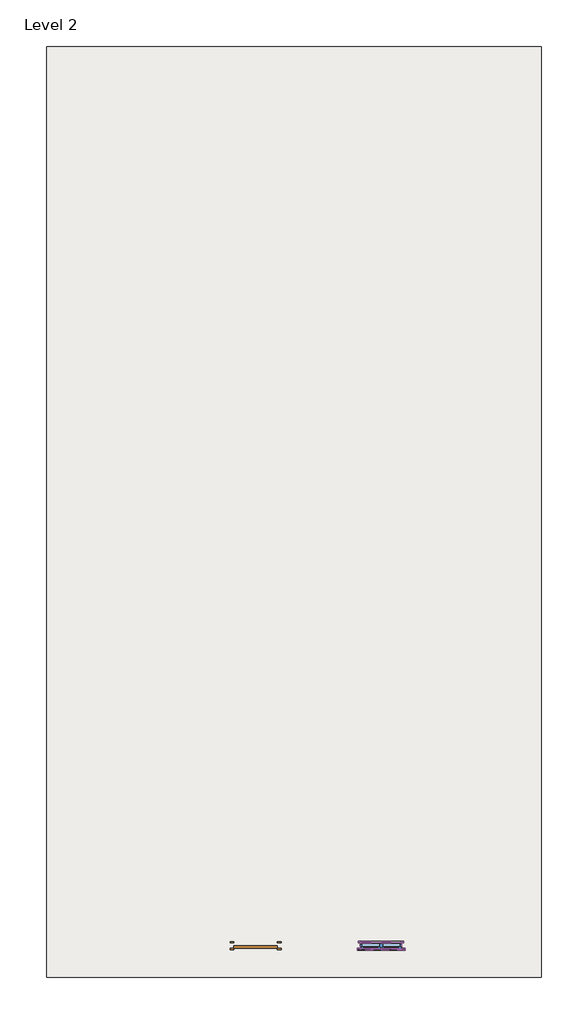
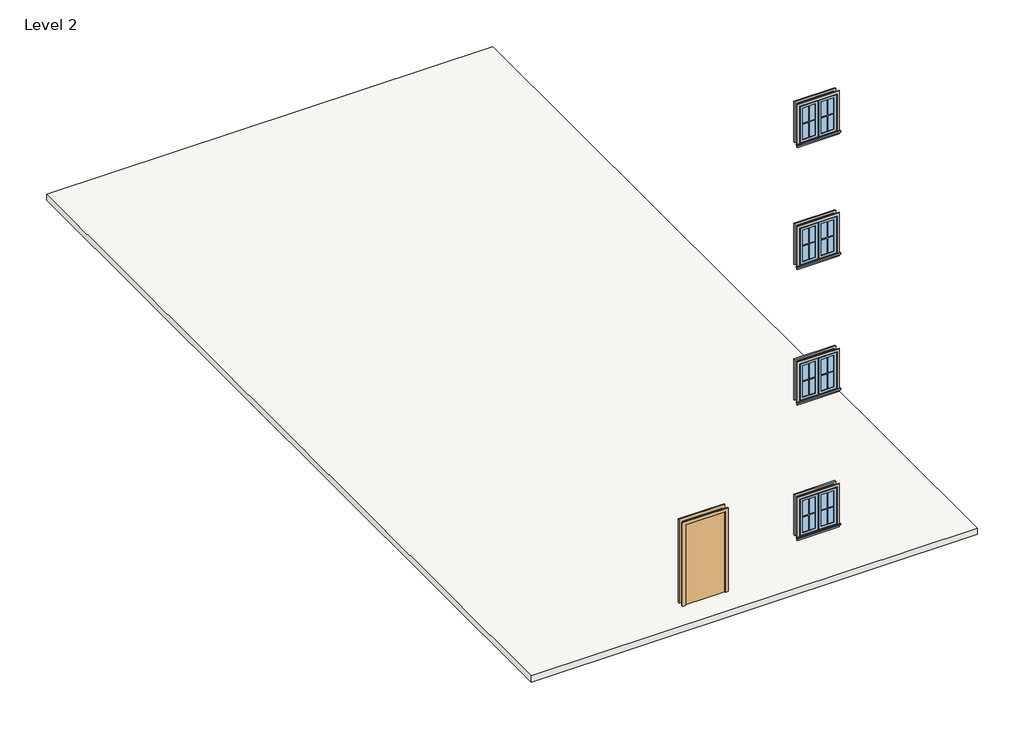
# One storey, incomplete: 16 proxies, 4 windows, 1 door, 1 roof.
"""IFC4 building model written with IfcOpenShell, lengths in millimetres."""

from ifc_helpers import new_model, si_unit, frame, origin, place, context, project, spatial, polyline, outline, extrude, transform, mapped, element, save
from components import muntin_pattern_2x2_muntin_pattern_2x2_b3fe6957, muntin_pattern_2x2_muntin_pattern_2x2_3e0ecaf2, trim_window_exterior_flat_with_sill_41619996, trim_window_interior_flat_picture_frame_51c85655, door_e5f9f3c4, window_a598f463

model = new_model("IFC4")

# Units and contexts
model_context = context("Model", 3, world=origin())
ifc_project = project(units=[si_unit("LENGTHUNIT", "METRE", prefix="MILLI")], contexts=[model_context])

# Site, building, storey
site = spatial("IfcSite", under=ifc_project)
building = spatial("IfcBuilding", under=site)
storey = spatial("IfcBuildingStorey", under=building, Name="Level 2", Elevation=3048.0)

# Proxies
placement = place(None, origin())
muntin_pattern_2x2_muntin_pattern_2x2_shape = muntin_pattern_2x2_muntin_pattern_2x2_b3fe6957(model_context)
element("IfcBuildingElementProxy", 1, Name="Muntin Pattern_2x2 : Muntin Pattern_2x2", ObjectType="Muntin Pattern_2x2 : Muntin Pattern_2x2", at=placement, inside=storey, context=model_context, shape_type="MappedRepresentation", body=[
    mapped(muntin_pattern_2x2_muntin_pattern_2x2_shape, transform((787.8709916, -7851.4177733, 4032.25), x_axis=(-1.0, 0.0, 0.0), y_axis=(0.0, -1.0, 0.0), z_axis=(0.0, 0.0, 1.0))),
])
element("IfcBuildingElementProxy", 2, Name="Muntin Pattern_2x2 : Muntin Pattern_2x2", ObjectType="Muntin Pattern_2x2 : Muntin Pattern_2x2", at=placement, inside=storey, context=model_context, shape_type="MappedRepresentation", body=[
    mapped(muntin_pattern_2x2_muntin_pattern_2x2_shape, transform((787.8709916, -7851.4177733, 7355.1690366), x_axis=(-1.0, 0.0, 0.0), y_axis=(0.0, -1.0, 0.0), z_axis=(0.0, 0.0, 1.0))),
])
element("IfcBuildingElementProxy", 3, Name="Muntin Pattern_2x2 : Muntin Pattern_2x2", ObjectType="Muntin Pattern_2x2 : Muntin Pattern_2x2", at=placement, inside=storey, context=model_context, shape_type="MappedRepresentation", body=[
    mapped(muntin_pattern_2x2_muntin_pattern_2x2_shape, transform((787.8709916, -7851.4177733, 10685.2522943), x_axis=(-1.0, 0.0, 0.0), y_axis=(0.0, -1.0, 0.0), z_axis=(0.0, 0.0, 1.0))),
])
element("IfcBuildingElementProxy", 4, Name="Muntin Pattern_2x2 : Muntin Pattern_2x2", ObjectType="Muntin Pattern_2x2 : Muntin Pattern_2x2", at=placement, inside=storey, context=model_context, shape_type="MappedRepresentation", body=[
    mapped(muntin_pattern_2x2_muntin_pattern_2x2_shape, transform((787.8709916, -7851.4177733, 13681.7979476), x_axis=(-1.0, 0.0, 0.0), y_axis=(0.0, -1.0, 0.0), z_axis=(0.0, 0.0, 1.0))),
])
muntin_pattern_2x2_muntin_pattern_2x2_2_shape = muntin_pattern_2x2_muntin_pattern_2x2_3e0ecaf2(model_context)
element("IfcBuildingElementProxy", 5, Name="Muntin Pattern_2x2 : Muntin Pattern_2x2", ObjectType="Muntin Pattern_2x2 : Muntin Pattern_2x2", at=placement, inside=storey, context=model_context, shape_type="MappedRepresentation", body=[
    mapped(muntin_pattern_2x2_muntin_pattern_2x2_2_shape, transform((359.2459916, -7851.4177733, 4032.25), x_axis=(1.0, 0.0, 0.0), y_axis=(0.0, 1.0, 0.0), z_axis=(0.0, 0.0, 1.0))),
])
element("IfcBuildingElementProxy", 6, Name="Muntin Pattern_2x2 : Muntin Pattern_2x2", ObjectType="Muntin Pattern_2x2 : Muntin Pattern_2x2", at=placement, inside=storey, context=model_context, shape_type="MappedRepresentation", body=[
    mapped(muntin_pattern_2x2_muntin_pattern_2x2_2_shape, transform((359.2459916, -7851.4177733, 7355.1690366), x_axis=(1.0, 0.0, 0.0), y_axis=(0.0, 1.0, 0.0), z_axis=(0.0, 0.0, 1.0))),
])
element("IfcBuildingElementProxy", 7, Name="Muntin Pattern_2x2 : Muntin Pattern_2x2", ObjectType="Muntin Pattern_2x2 : Muntin Pattern_2x2", at=placement, inside=storey, context=model_context, shape_type="MappedRepresentation", body=[
    mapped(muntin_pattern_2x2_muntin_pattern_2x2_2_shape, transform((359.2459916, -7851.4177733, 10685.2522943), x_axis=(1.0, 0.0, 0.0), y_axis=(0.0, 1.0, 0.0), z_axis=(0.0, 0.0, 1.0))),
])
element("IfcBuildingElementProxy", 8, Name="Muntin Pattern_2x2 : Muntin Pattern_2x2", ObjectType="Muntin Pattern_2x2 : Muntin Pattern_2x2", at=placement, inside=storey, context=model_context, shape_type="MappedRepresentation", body=[
    mapped(muntin_pattern_2x2_muntin_pattern_2x2_2_shape, transform((359.2459916, -7851.4177733, 13681.7979476), x_axis=(1.0, 0.0, 0.0), y_axis=(0.0, 1.0, 0.0), z_axis=(0.0, 0.0, 1.0))),
])
trim_window_exterior_flat_with_sill_shape = trim_window_exterior_flat_with_sill_41619996(model_context)
element("IfcBuildingElementProxy", 9, Name="Trim-Window-Exterior-Flat : with Sill", ObjectType="Trim-Window-Exterior-Flat : with Sill", at=placement, inside=storey, context=model_context, shape_type="MappedRepresentation", body=[
    mapped(trim_window_exterior_flat_with_sill_shape, transform((573.5584916, -7860.9427733, 4876.8), x_axis=(1.0, 0.0, 0.0), y_axis=(0.0, 0.0, 1.0), z_axis=(0.0, -1.0, 0.0))),
])
element("IfcBuildingElementProxy", 10, Name="Trim-Window-Exterior-Flat : with Sill", ObjectType="Trim-Window-Exterior-Flat : with Sill", at=placement, inside=storey, context=model_context, shape_type="MappedRepresentation", body=[
    mapped(trim_window_exterior_flat_with_sill_shape, transform((573.5584916, -7860.9427733, 8199.7190366), x_axis=(1.0, 0.0, 0.0), y_axis=(0.0, 0.0, 1.0), z_axis=(0.0, -1.0, 0.0))),
])
element("IfcBuildingElementProxy", 11, Name="Trim-Window-Exterior-Flat : with Sill", ObjectType="Trim-Window-Exterior-Flat : with Sill", at=placement, inside=storey, context=model_context, shape_type="MappedRepresentation", body=[
    mapped(trim_window_exterior_flat_with_sill_shape, transform((573.5584916, -7860.9427733, 11529.8022943), x_axis=(1.0, 0.0, 0.0), y_axis=(0.0, 0.0, 1.0), z_axis=(0.0, -1.0, 0.0))),
])
element("IfcBuildingElementProxy", 12, Name="Trim-Window-Exterior-Flat : with Sill", ObjectType="Trim-Window-Exterior-Flat : with Sill", at=placement, inside=storey, context=model_context, shape_type="MappedRepresentation", body=[
    mapped(trim_window_exterior_flat_with_sill_shape, transform((573.5584916, -7860.9427733, 14526.3479476), x_axis=(1.0, 0.0, 0.0), y_axis=(0.0, 0.0, 1.0), z_axis=(0.0, -1.0, 0.0))),
])
trim_window_interior_flat_picture_frame_shape = trim_window_interior_flat_picture_frame_51c85655(model_context)
element("IfcBuildingElementProxy", 13, Name="Trim-Window-Interior-Flat : Picture Frame", ObjectType="Trim-Window-Interior-Flat : Picture Frame", at=placement, inside=storey, context=model_context, shape_type="MappedRepresentation", body=[
    mapped(trim_window_interior_flat_picture_frame_shape, transform((573.5584916, -7746.6427733, 4876.8), x_axis=(-1.0, 0.0, 0.0), y_axis=(0.0, 0.0, 1.0), z_axis=(0.0, 1.0, 0.0))),
])
element("IfcBuildingElementProxy", 14, Name="Trim-Window-Interior-Flat : Picture Frame", ObjectType="Trim-Window-Interior-Flat : Picture Frame", at=placement, inside=storey, context=model_context, shape_type="MappedRepresentation", body=[
    mapped(trim_window_interior_flat_picture_frame_shape, transform((573.5584916, -7746.6427733, 8199.7190366), x_axis=(-1.0, 0.0, 0.0), y_axis=(0.0, 0.0, 1.0), z_axis=(0.0, 1.0, 0.0))),
])
element("IfcBuildingElementProxy", 15, Name="Trim-Window-Interior-Flat : Picture Frame", ObjectType="Trim-Window-Interior-Flat : Picture Frame", at=placement, inside=storey, context=model_context, shape_type="MappedRepresentation", body=[
    mapped(trim_window_interior_flat_picture_frame_shape, transform((573.5584916, -7746.6427733, 11529.8022943), x_axis=(-1.0, 0.0, 0.0), y_axis=(0.0, 0.0, 1.0), z_axis=(0.0, 1.0, 0.0))),
])
element("IfcBuildingElementProxy", 16, Name="Trim-Window-Interior-Flat : Picture Frame", ObjectType="Trim-Window-Interior-Flat : Picture Frame", at=placement, inside=storey, context=model_context, shape_type="MappedRepresentation", body=[
    mapped(trim_window_interior_flat_picture_frame_shape, transform((573.5584916, -7746.6427733, 14526.3479476), x_axis=(-1.0, 0.0, 0.0), y_axis=(0.0, 0.0, 1.0), z_axis=(0.0, 1.0, 0.0))),
])

# Door
door_shape = door_e5f9f3c4(model_context)
element("IfcDoor", 17, ObjectType="Single-Flush : 36\" x 84\"", at=placement, inside=storey, context=model_context, shape_type="MappedRepresentation", body=[
    mapped(door_shape, transform((-2055.3415084, -7803.7927733, 3048.0), x_axis=(-1.0, 0.0, 0.0), y_axis=(0.0, -1.0, 0.0), z_axis=(0.0, 0.0, 1.0))),
])

# Roof
element("IfcRoof", 18, ObjectType="Generic - 12\"", at=placement, inside=storey, context=model_context, shape_type="SweptSolid", body=[
    extrude(outline(polyline([(-6436.8415084, 11036.6572267), (3926.3584916, 11036.6572267), (3926.3584916, -8470.5427733), (-6436.8415084, -8470.5427733), (-6436.8415084, 11036.6572267)])), frame((0.0, 0.0, 3048.0), z_axis=(0.0, 0.0, 1.0), x_axis=(1.0, 0.0, 0.0)), (0.0, 0.0, 1.0), 152.4),
])

# Windows
window_shape = window_a598f463(model_context)
element("IfcWindow", 19, ObjectType="Window-Casement-Double : 34\" x 36\"", at=placement, inside=storey, context=model_context, shape_type="MappedRepresentation", body=[
    mapped(window_shape, transform((573.5584916, -7803.7927733, 3048.0), x_axis=(-1.0, 0.0, 0.0), y_axis=(0.0, -1.0, 0.0), z_axis=(0.0, 0.0, 1.0))),
])
element("IfcWindow", 20, ObjectType="Window-Casement-Double : 34\" x 36\"", at=placement, inside=storey, context=model_context, shape_type="MappedRepresentation", body=[
    mapped(window_shape, transform((573.5584916, -7803.7927733, 6370.9190366), x_axis=(-1.0, 0.0, 0.0), y_axis=(0.0, -1.0, 0.0), z_axis=(0.0, 0.0, 1.0))),
])
element("IfcWindow", 21, ObjectType="Window-Casement-Double : 34\" x 36\"", at=placement, inside=storey, context=model_context, shape_type="MappedRepresentation", body=[
    mapped(window_shape, transform((573.5584916, -7803.7927733, 9701.0022943), x_axis=(-1.0, 0.0, 0.0), y_axis=(0.0, -1.0, 0.0), z_axis=(0.0, 0.0, 1.0))),
])
element("IfcWindow", 22, ObjectType="Window-Casement-Double : 34\" x 36\"", at=placement, inside=storey, context=model_context, shape_type="MappedRepresentation", body=[
    mapped(window_shape, transform((573.5584916, -7803.7927733, 12697.5479476), x_axis=(-1.0, 0.0, 0.0), y_axis=(0.0, -1.0, 0.0), z_axis=(0.0, 0.0, 1.0))),
])

save(model, "model.ifc")

# Revit data of these elements
# Type "Muntin Pattern_2x2 : Muntin Pattern_2x2"
#   Width [instance default] = 4' - 0"
#   Thickness = 0' - 0 1/2"
#   Height [instance default] = 4' - 0"
#   Distance = 0' - 0 3/4"
#   Interior Material [instance default] = none
#   Exterior Material [instance default] = none
#   Default Elevation = 0
# Type "Trim-Window-Exterior-Flat : with Sill"
#   Trim Width = 0' - 2 1/4"
#   Trim Thickness_Picture Frame = 0' - 1 1/4"
#   Trim Thickness_with Sill = 0' - 0 3/4"
#   Sill Thickness = 0' - 1 1/4"
#   Opening Width [instance default] = 2' - 0"
#   Opening Height [instance default] = 3' - 0"
#   Default Elevation = 4' - 0"
#   Sill = yes
#   Picture Frame = no
#   Trim Material [instance default] = none
# Type "Trim-Window-Interior-Flat : Picture Frame"
#   Trim Thickness_Picture Frame = 0' - 1 1/4"
#   Trim Width = 0' - 2 1/4"
#   Trim Thickness_with Sill = 0' - 0 3/4"
#   Sill Thickness = 0' - 1 1/4"
#   Opening Width [instance default] = 2' - 0"
#   Opening Height [instance default] = 3' - 0"
#   Default Elevation = 4' - 0"
#   Sill = no
#   Picture Frame = yes
#   Trim Material [instance default] = none
# Type "Single-Flush : 36\" x 84\""
#   Type Mark = "1"
#   Construction Type Id = "MDOOR"
#   Assembly Code = "C1020"
#   Analytic Construction = "Metal"
#   Thickness = 0' - 2"
#   Heat Transfer Coefficient (U) = 0.651978 BTU/(h·ft²·°F)
#   Height = 7' - 0"
#   Trim Projection Ext = 0' - 1"
#   Trim Projection Int = 0' - 1"
#   Trim Width = 0' - 3"
#   Width = 3' - 0"
#   Define Thermal Properties by = 1
#   Define Thermal Properties by = 1
#   Door Material = Door - Panel
#   Frame Material = Door - Frame
#   Visual Light Transmittance = 0
#   Solar Heat Gain Coefficient = 0
#   Function = (empty or 0)
#   Wall Closure = (empty or 0)
# Type "Generic - 12\""
#   Assembly Code = "B1020"
#   Layers, outside or top first: 0' - 6" no material (function 1)
# Type "Window-Casement-Double : 34\" x 36\""
#   Type Mark = "14"
#   Fire Rating = "0.5h"
#   Assembly Code = "B2020100"
#   Analytic Construction = "Double glazing - domestic"
#   Frame Extension [instance default] = 0' - 0 1/4"
#   Window Inset [instance default] = 0' - 0"
#   Wall Thickness [instance default] = 0' - 6"
#   Interior Wall Closure [instance default] = 0' - 2 1/4"
#   Half Width = 1' - 5"
#   Visual Light Transmittance = 0.81
#   Thermal Resistance (R) = 1.8146 (h·ft²·°F)/BTU
#   Solar Heat Gain Coefficient = 0.76
#   Rough Width = 2' - 10 1/2"
#   Rough Height = 3' - 0 1/2"
#   Height = 3' - 0"
#   Heat Transfer Coefficient (U) = 0.5511 BTU/(h·ft²·°F)
#   Exterior Wall Closure [instance default] = 0' - 1 1/4"
#   Extension Jamb [instance default] = 0' - 2 1/4"
#   Default Sill Height = 3' - 0"
#   Width = 2' - 10"
#   Define Thermal Properties by = 0
#   Muntin Visibility = yes
#   Interior Trim Visibility [instance default] = yes
#   Exterior Trim Visibility [instance default] = yes
#   Extension Jamb Visibility [instance default] = yes
#   Interior Trim Material = Wood - Stained
#   Muntin Pattern = Muntin Pattern_2x2 : Muntin Pattern_2x2
#   Interior Trim = Trim-Window-Interior-Flat : Picture Frame
#   Interior Frame Material = Wood - Stained
#   Glass Panel Material = Glass
#   Exterior Trim Material = Clad - White
#   Exterior Trim = Trim-Window-Exterior-Flat : with Sill
#   Exterior Frame Material = Clad - White
#   Wall Closure = (empty or 0)
# Elements 1, 2, 3, 4, 5, 6, 7, 8 (IfcBuildingElementProxy, "Muntin Pattern_2x2 : Muntin Pattern_2x2")
#   Width = 0' - 11 5/8"
#   Height = 2' - 6 1/2"
#   Interior Material = Wood - Stained
#   Exterior Material = Clad - White
#   Phase Created = New Construction
#   Materials on its faces: "Clad - White", "Wood - Stained"
# Elements 9, 10, 11, 12 (IfcBuildingElementProxy, "Trim-Window-Exterior-Flat : with Sill")
#   Opening Width = 2' - 10"
#   Opening Height = 3' - 0"
#   Trim Material = Clad - White
#   Phase Created = New Construction
#   Materials on its faces: "Clad - White"
# Elements 13, 14, 15, 16 (IfcBuildingElementProxy, "Trim-Window-Interior-Flat : Picture Frame")
#   Opening Width = 2' - 10"
#   Opening Height = 3' - 0"
#   Trim Material = Wood - Stained
#   Phase Created = New Construction
#   Materials on its faces: "Wood - Stained"
# Element 17 (IfcDoor, "Single-Flush : 36\" x 84\"")
#   Phase Created = New Construction
#   Materials on its faces: "Door - Frame", "Door - Panel"
# Element 18 (IfcRoof, "Generic - 12\"")
#   built-in parameter 1001705 = 10.5 (stored number, unit not read)
#   built-in parameter 1001710 = 33615
#   Phase Created = New Construction
#   Materials on its faces: "Default Roof", "Wood Planks"
# Element 19 (IfcWindow, "Window-Casement-Double : 34\" x 36\"")
#   Mark = "46"
#   Window Inset = 0' - 0"
#   Interior Wall Closure = 0' - 2 1/4"
#   Frame Extension = 0' - 0 1/4"
#   Exterior Wall Closure = 0' - 1 1/4"
#   Interior Trim Visibility = yes
#   Exterior Trim Visibility = yes
#   Phase Created = New Construction
#   Materials on its faces: "Wood - Stained", "Glass", "Clad - White"
# Element 20 (IfcWindow, "Window-Casement-Double : 34\" x 36\"")
#   Mark = "47"
#   Window Inset = 0' - 0"
#   Interior Wall Closure = 0' - 2 1/4"
#   Frame Extension = 0' - 0 1/4"
#   Exterior Wall Closure = 0' - 1 1/4"
#   Interior Trim Visibility = yes
#   Exterior Trim Visibility = yes
#   Phase Created = New Construction
#   Materials on its faces: "Wood - Stained", "Glass", "Clad - White"
# Element 21 (IfcWindow, "Window-Casement-Double : 34\" x 36\"")
#   Mark = "48"
#   Window Inset = 0' - 0"
#   Interior Wall Closure = 0' - 2 1/4"
#   Frame Extension = 0' - 0 1/4"
#   Exterior Wall Closure = 0' - 1 1/4"
#   Interior Trim Visibility = yes
#   Exterior Trim Visibility = yes
#   Phase Created = New Construction
#   Materials on its faces: "Wood - Stained", "Glass", "Clad - White"
# Element 22 (IfcWindow, "Window-Casement-Double : 34\" x 36\"")
#   Mark = "49"
#   Window Inset = 0' - 0"
#   Interior Wall Closure = 0' - 2 1/4"
#   Frame Extension = 0' - 0 1/4"
#   Exterior Wall Closure = 0' - 1 1/4"
#   Interior Trim Visibility = yes
#   Exterior Trim Visibility = yes
#   Phase Created = New Construction
#   Materials on its faces: "Wood - Stained", "Glass", "Clad - White"
# Materials
#   "Door - Panel": class "Wood", colour RGB 210 159 95, transparency 0, Cost = 0
#   "Door - Frame": colour RGB 118 70 51, transparency 0, Cost = 0
#   "Wood - Stained": class "Wood", colour RGB 224 178 126, transparency 0, Cost = 0
#   "Glass": class "Glass", colour RGB 0 128 192, transparency 0.75, Description = "Soda Lime Glass", Cost = 0
#   "Clad - White": class "Wood", colour RGB 242 242 238, transparency 0, Cost = 0
#   "Default Roof": colour RGB 88 101 114, transparency 0, Cost = 0
#   "Wood Planks": class "Wood", colour RGB 193 160 115, transparency 0, Description = "Physical material.", Cost = 0
